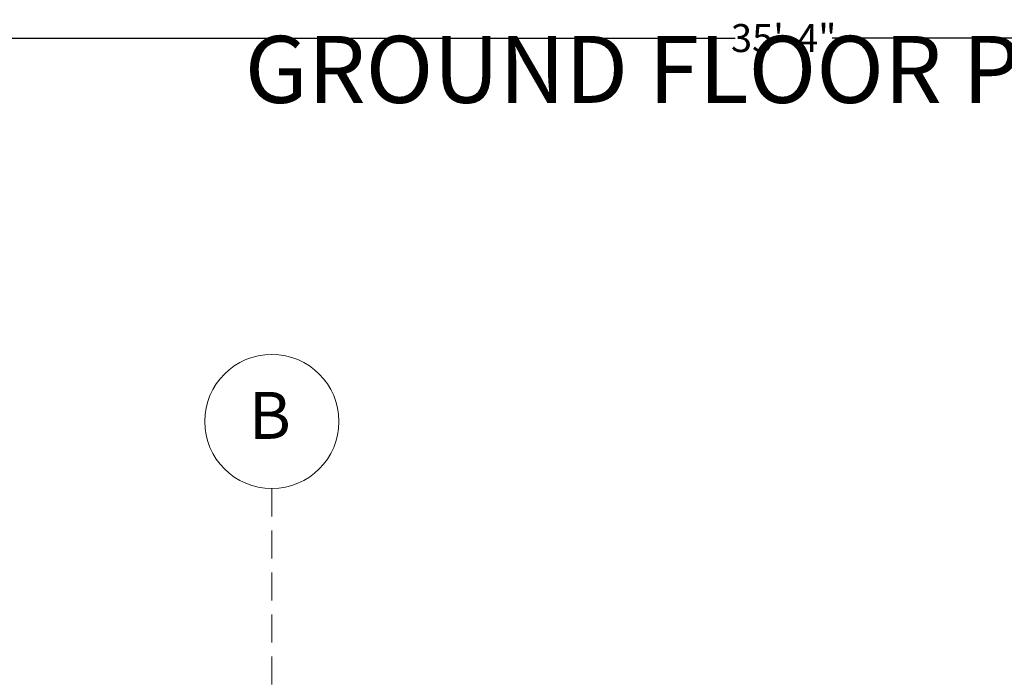
# Model space of a CAD drawing. Units: inches. Extents: x 782 to 2660, y -1008 to 166.
# Tile 9 of 12: x 1058 to 1234, y 48 to 166. Entities that reach past the tile are written whole.
import ezdxf

# ---------------------------------------------------------------- set-up
doc = ezdxf.new("R2010")
doc.units = ezdxf.units.IN
doc.header["$MEASUREMENT"] = 0
doc.linetypes.add('DASHED', pattern=[0.75, 0.5, -0.25])
for name, color, linetype, lineweight in [('A-ANNO-DIMS', 4, 'Continuous', 18), ('A-ANNO-TEXT', 4, 'Continuous', 18), ('A-GRID', 8, 'DASHED', 13), ('A-GRID-IDEN', 7, 'Continuous', 18)]:
    doc.layers.add(name, color=color, linetype=linetype, lineweight=lineweight)
doc.styles.get("Standard").update_dxf_attribs({"font": 'arial.ttf'})
doc.dimstyles.get("Standard").update_dxf_attribs({"dimtxt": 5, "dimasz": 2, "dimexe": 0.18, "dimexo": 0.0625, "dimgap": 0.09, "dimtad": 0, "dimtih": 1, "dimtoh": 1, "dimdec": 0, "dimzin": 0, "dimdsep": 46, "dimlunit": 3, "dimtxsty": 'Standard', "dimblk": 'ARCHTICK', "dimcen": 0.09, "dimadec": 0, "dimazin": 0, "dimtfac": 1, "dimtdec": 0, "dimtofl": 0, "dimtmove": 0, "dimatfit": 3, "dimfxl": 1, "dimtolj": 1, "dimtzin": 0, "dimarcsym": 0})

# ---------------------------------------------------------------- blocks, each defined once
blk = doc.blocks.new('_ArchTick')
at = {"color": 0, "linetype": 'ByBlock', "const_width": 0.15}
blk.add_lwpolyline([(-0.5, -0.5), (0.5, 0.5)], dxfattribs=at)
blk = doc.blocks.new('*D52')
at = {"layer": 'A-ANNO-DIMS', "color": 0, "lineweight": -2, "transparency": 16777216}
for p, q in [((982.68, 45.07), (982.68, 163.27)), ((982.68, 163.09), (1186.01, 163.09)), ((1406.68, 163.09), (1203.36, 163.09)), ((1406.68, 45.07), (1406.68, 163.27))]:
    blk.add_line(p, q, dxfattribs=at)
at = {"layer": 'Defpoints', "color": 0, "transparency": 16777216}
for p in [(1406.68, 163.09), (982.68, 45.01), (1406.68, 45.01)]:
    blk.add_point(p, dxfattribs=at)
at = {"layer": 'A-ANNO-DIMS', "color": 0, "lineweight": -2, "transparency": 16777216, "xscale": 2, "yscale": 2, "zscale": 2, "rotation": 180}
blk.add_blockref('_ArchTick', (982.68, 163.09), dxfattribs=at)
at = {"layer": 'A-ANNO-DIMS', "color": 0, "lineweight": -2, "transparency": 16777216, "xscale": 2, "yscale": 2, "zscale": 2}
blk.add_blockref('_ArchTick', (1406.68, 163.09), dxfattribs=at)
at = {"layer": 'A-ANNO-DIMS', "color": 0, "transparency": 16777216, "insert": (1194.68, 163.09), "char_height": 5, "attachment_point": 5}
blk.add_mtext('\\A1;35\'-4"', dxfattribs=at)

msp = doc.modelspace()

# ---------------------------------------------------------------- linework, layer by layer
at = {"layer": 'A-GRID', "ltscale": 10}
msp.add_line((1103.18, 82.53), (1103.18, -946.37), dxfattribs=at)
at = {"layer": 'A-GRID-IDEN'}
msp.add_circle((1103.18, 94.53), 12, dxfattribs=at)

# ---------------------------------------------------------------- texts
at = {"layer": 'A-ANNO-TEXT'}
msp.add_text('GROUND FLOOR PLAN', height=11.9654, dxfattribs=at).set_placement((1098.34, 151.5))
at = {"layer": 'A-GRID-IDEN'}
msp.add_text('B', height=8.41, dxfattribs=at).set_placement((1099.05, 91.42))

# ---------------------------------------------------------------- dimensions: what is measured, and where the dimension line sits
at = {"layer": 'A-ANNO-DIMS'}
dim = msp.add_linear_dim(base=(1406.68, 163.09), p1=(982.68, 45.01), p2=(1406.68, 45.01), dimstyle='Standard', override={"dimdec": 1, "dimlfac": 1, "dimrnd": 0, "dimzin": 1, "dimdsep": 46, "dimlunit": 4, "dimfrac": 2}, dxfattribs=at)
dim.commit()
dim.dimension.update_dxf_attribs({"geometry": '*D52', "text_midpoint": (1194.68, 163.09)})

doc.saveas('drawing.dxf')
